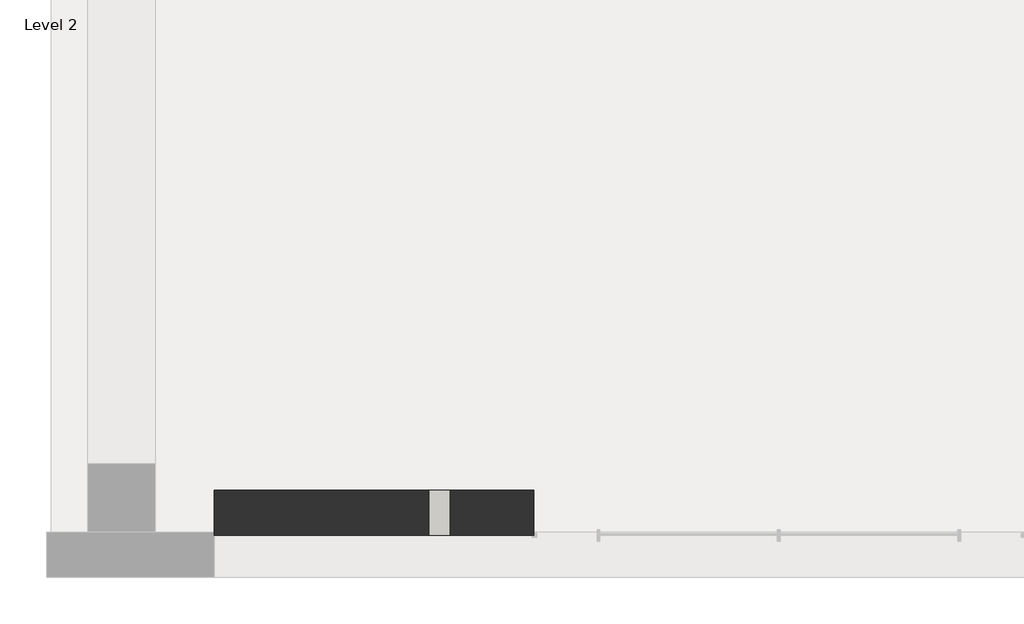
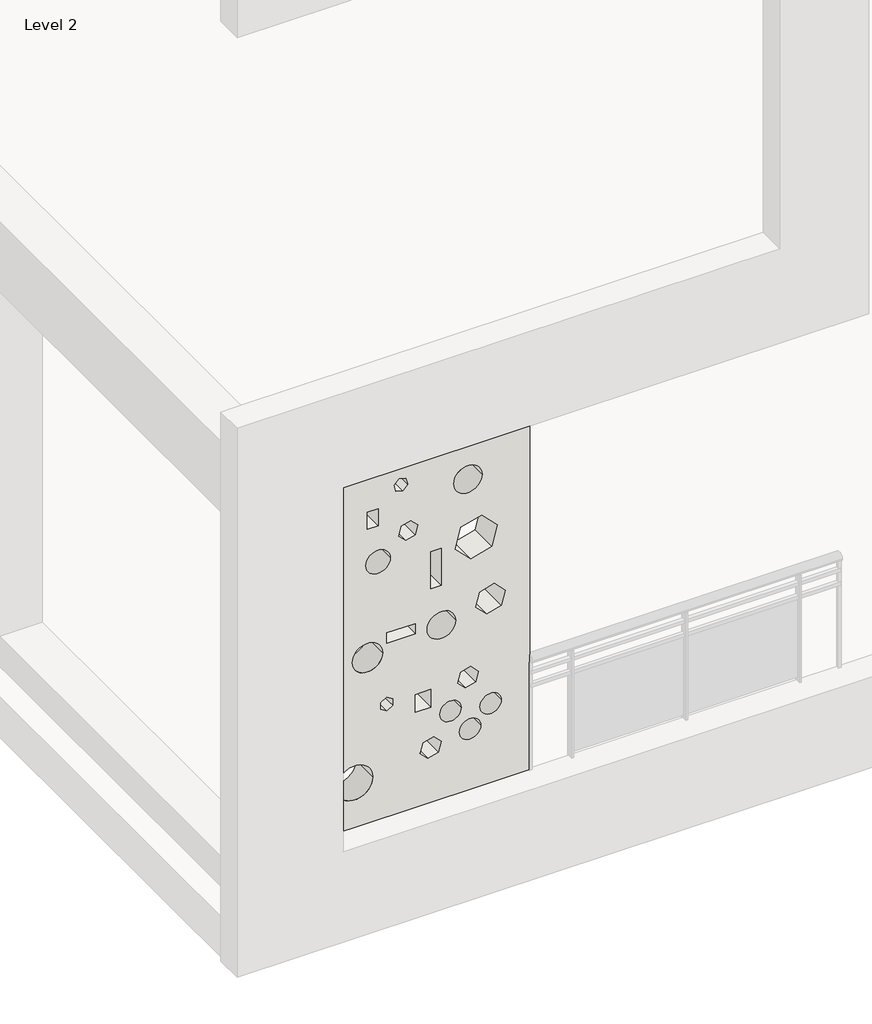
# One storey, part 1 of 2: 1 wall.
"""IFC4 building model written with IfcOpenShell, lengths in millimetres."""

from ifc_helpers import new_model, si_unit, frame, origin, place, context, project, spatial, polyline, circle_curve, element, save
from ifc_brep_helpers import plane_surface, revolved_surface, advanced_brep

model = new_model("IFC4")

# Units and contexts
model_context = context("Model", 3, world=origin())
ifc_project = project(units=[si_unit("LENGTHUNIT", "METRE", prefix="MILLI")], contexts=[model_context])

# Site, building, storey
site = spatial("IfcSite", under=ifc_project)
building = spatial("IfcBuilding", under=site)
storey = spatial("IfcBuildingStorey", under=building, Name="Level 2", Elevation=3657.6)

# Wall
placement = place(None, origin())
element("IfcWall", 1, ObjectType="Generic - 8\"", at=placement, inside=storey, context=model_context, shape_type="AdvancedBrep", body=[
    advanced_brep(
    [(-10102.8741466, 1544.2572776, 4341.7312703), (-8663.1307892, 1544.2572776, 4341.7312703), (-8663.1307892, 1544.2572776, 7084.9312703), (-10102.8741466, 1544.2572776, 7084.9312703), (-9743.8434722, 1544.2572776, 6685.8043423), (-9743.8434722, 1544.2572776, 6558.8043423), (-9820.0434722, 1544.2572776, 6558.8043423), (-9820.0434722, 1544.2572776, 6685.8043423), (-9292.3903484, 1544.2572776, 6229.9318449), (-9292.3903484, 1544.2572776, 5950.5318449), (-9368.5903484, 1544.2572776, 5950.5318449), (-9368.5903484, 1544.2572776, 6229.9318449), (-9479.1821198, 1544.2572776, 5728.8819866), (-9479.1821198, 1544.2572776, 5652.6819866), (-9682.3821198, 1544.2572776, 5652.6819866), (-9682.3821198, 1544.2572776, 5728.8819866), (-9368.5903484, 1544.2572776, 5193.0240889), (-9368.5903484, 1544.2572776, 5060.1832779), (-9479.1821198, 1544.2572776, 5060.1832779), (-9479.1821198, 1544.2572776, 5193.0240889), (-9001.4296873, 1544.2572776, 6685.8043423), (-9204.6296873, 1544.2572776, 6685.8043423), (-9656.9239941, 1544.2572776, 6287.1198438), (-9830.7629503, 1544.2572776, 6287.1198438), (-9190.7903484, 1544.2572776, 5652.6819866), (-9393.9903484, 1544.2572776, 5652.6819866), (-8970.421925, 1544.2572776, 5624.7908508), (-9046.621925, 1544.2572776, 5700.9908508), (-9018.7307892, 1544.2572776, 5805.0819866), (-8914.6396534, 1544.2572776, 5832.9731223), (-8838.4396534, 1544.2572776, 5756.7731223), (-8866.3307892, 1544.2572776, 5652.6819866), (-9084.3253885, 1544.2572776, 6079.9235581), (-9194.1390761, 1544.2572776, 6189.7372456), (-9153.9444768, 1544.2572776, 6339.7455325), (-9003.9361899, 1544.2572776, 6379.9401318), (-8894.1225023, 1544.2572776, 6270.1264443), (-8934.3171017, 1544.2572776, 6120.1181574), (-9630.1079092, 1544.2572776, 6823.2802275), (-9594.1868847, 1544.2572776, 6859.2012519), (-9545.1178527, 1544.2572776, 6846.0532445), (-9531.9698452, 1544.2572776, 6796.9842125), (-9567.8908697, 1544.2572776, 6761.063188), (-9616.9599017, 1544.2572776, 6774.2111955), (-9547.9311575, 1544.2572776, 6379.0943395), (-9598.2589461, 1544.2572776, 6429.4221281), (-9579.837697, 1544.2572776, 6498.1711658), (-9511.0886592, 1544.2572776, 6516.592415), (-9460.7608706, 1544.2572776, 6466.2646264), (-9479.1821198, 1544.2572776, 6397.5155887), (-9726.3762103, 1544.2572776, 5167.6240889), (-9726.3762103, 1544.2572776, 5218.4240889), (-9682.3821198, 1544.2572776, 5243.8240889), (-9638.3880293, 1544.2572776, 5218.4240889), (-9638.3880293, 1544.2572776, 5167.6240889), (-9682.3821198, 1544.2572776, 5142.2240889), (-9121.9120367, 1544.2572776, 5119.4205409), (-9175.7935734, 1544.2572776, 5173.3020776), (-9156.0715622, 1544.2572776, 5246.9056256), (-9082.4680142, 1544.2572776, 5266.6276368), (-9028.5864775, 1544.2572776, 5212.7461001), (-9048.3084887, 1544.2572776, 5139.1425521), (-9388.391626, 1544.2572776, 4681.4839037), (-9442.4897226, 1544.2572776, 4735.5820003), (-9422.688445, 1544.2572776, 4809.4813745), (-9348.7890707, 1544.2572776, 4829.2826522), (-9294.6909741, 1544.2572776, 4775.1845556), (-9314.4922518, 1544.2572776, 4701.2851813), (-9011.4676213, 1544.2572776, 4798.8655131), (-9163.8676213, 1544.2572776, 4798.8655131), (-8864.8322569, 1544.2572776, 4938.5407612), (-9017.2322569, 1544.2572776, 4938.5407612), (-9151.0988797, 1544.2572776, 4981.0816577), (-9303.4988797, 1544.2572776, 4981.0816577), (-9782.375451, 1544.2572776, 4678.6434787), (-10039.5887886, 1544.2572776, 4678.6434787), (-9712.2803987, 1544.2572776, 5590.3709003), (-9927.8065456, 1544.2572776, 5590.3709003), (-10102.8741466, 1747.4572776, 4341.7312703), (-10102.8741466, 1747.4572776, 7084.9312703), (-8663.1307892, 1747.4572776, 7084.9312703), (-8663.1307892, 1747.4572776, 4341.7312703), (-9743.8434722, 1747.4572776, 6685.8043423), (-9820.0434722, 1747.4572776, 6685.8043423), (-9820.0434722, 1747.4572776, 6558.8043423), (-9743.8434722, 1747.4572776, 6558.8043423), (-9292.3903484, 1747.4572776, 6229.9318449), (-9368.5903484, 1747.4572776, 6229.9318449), (-9368.5903484, 1747.4572776, 5950.5318449), (-9292.3903484, 1747.4572776, 5950.5318449), (-9479.1821198, 1747.4572776, 5728.8819866), (-9682.3821198, 1747.4572776, 5728.8819866), (-9682.3821198, 1747.4572776, 5652.6819866), (-9479.1821198, 1747.4572776, 5652.6819866), (-9368.5903484, 1747.4572776, 5193.0240889), (-9479.1821198, 1747.4572776, 5193.0240889), (-9479.1821198, 1747.4572776, 5060.1832779), (-9368.5903484, 1747.4572776, 5060.1832779), (-9001.4296873, 1747.4572776, 6685.8043423), (-9204.6296873, 1747.4572776, 6685.8043423), (-9656.9239941, 1747.4572776, 6287.1198438), (-9830.7629503, 1747.4572776, 6287.1198438), (-9190.7903484, 1747.4572776, 5652.6819866), (-9393.9903484, 1747.4572776, 5652.6819866), (-8970.421925, 1747.4572776, 5624.7908508), (-8866.3307892, 1747.4572776, 5652.6819866), (-8838.4396534, 1747.4572776, 5756.7731223), (-8914.6396534, 1747.4572776, 5832.9731223), (-9018.7307892, 1747.4572776, 5805.0819866), (-9046.621925, 1747.4572776, 5700.9908508), (-9084.3253885, 1747.4572776, 6079.9235581), (-8934.3171017, 1747.4572776, 6120.1181574), (-8894.1225023, 1747.4572776, 6270.1264443), (-9003.9361899, 1747.4572776, 6379.9401318), (-9153.9444768, 1747.4572776, 6339.7455325), (-9194.1390761, 1747.4572776, 6189.7372456), (-9630.1079092, 1747.4572776, 6823.2802275), (-9616.9599017, 1747.4572776, 6774.2111955), (-9567.8908697, 1747.4572776, 6761.063188), (-9531.9698452, 1747.4572776, 6796.9842125), (-9545.1178527, 1747.4572776, 6846.0532445), (-9594.1868847, 1747.4572776, 6859.2012519), (-9547.9311575, 1747.4572776, 6379.0943395), (-9479.1821198, 1747.4572776, 6397.5155887), (-9460.7608706, 1747.4572776, 6466.2646264), (-9511.0886592, 1747.4572776, 6516.592415), (-9579.837697, 1747.4572776, 6498.1711658), (-9598.2589461, 1747.4572776, 6429.4221281), (-9726.3762103, 1747.4572776, 5167.6240889), (-9682.3821198, 1747.4572776, 5142.2240889), (-9638.3880293, 1747.4572776, 5167.6240889), (-9638.3880293, 1747.4572776, 5218.4240889), (-9682.3821198, 1747.4572776, 5243.8240889), (-9726.3762103, 1747.4572776, 5218.4240889), (-9121.9120367, 1747.4572776, 5119.4205409), (-9048.3084887, 1747.4572776, 5139.1425521), (-9028.5864775, 1747.4572776, 5212.7461001), (-9082.4680142, 1747.4572776, 5266.6276368), (-9156.0715622, 1747.4572776, 5246.9056256), (-9175.7935734, 1747.4572776, 5173.3020776), (-9388.391626, 1747.4572776, 4681.4839037), (-9314.4922518, 1747.4572776, 4701.2851813), (-9294.6909741, 1747.4572776, 4775.1845556), (-9348.7890707, 1747.4572776, 4829.2826522), (-9422.688445, 1747.4572776, 4809.4813745), (-9442.4897226, 1747.4572776, 4735.5820003), (-9011.4676213, 1747.4572776, 4798.8655131), (-9163.8676213, 1747.4572776, 4798.8655131), (-8864.8322569, 1747.4572776, 4938.5407612), (-9017.2322569, 1747.4572776, 4938.5407612), (-9151.0988797, 1747.4572776, 4981.0816577), (-9303.4988797, 1747.4572776, 4981.0816577), (-9782.375451, 1747.4572776, 4678.6434787), (-10039.5887886, 1747.4572776, 4678.6434787), (-9712.2803987, 1747.4572776, 5590.3709003), (-9927.8065456, 1747.4572776, 5590.3709003), (-10102.8741466, 1558.4652184, 4341.7312703), (-10102.8741466, 1558.4652184, 7084.9312703)],
    [
        (0, 1),
        (1, 2),
        (2, 3),
        (3, 0),
        (4, 5),
        (5, 6),
        (6, 7),
        (7, 4),
        (8, 9),
        (9, 10),
        (10, 11),
        (11, 8),
        (12, 13),
        (13, 14),
        (14, 15),
        (15, 12),
        (16, 17),
        (17, 18),
        (18, 19),
        (19, 16),
        (20, 21, circle_curve(frame((-9103.0296873, 1544.2572776, 6685.8043423), z_axis=(0.0, 1.0, 0.0), x_axis=(-1.0, 0.0, 0.0)), 101.6)),
        (21, 20, circle_curve(frame((-9103.0296873, 1544.2572776, 6685.8043423), z_axis=(0.0, 1.0, 0.0), x_axis=(-1.0, 0.0, 0.0)), 101.6)),
        (22, 23, circle_curve(frame((-9743.8434722, 1544.2572776, 6287.1198438), z_axis=(0.0, 1.0, 0.0), x_axis=(-1.0, 0.0, 0.0)), 86.9194781)),
        (23, 22, circle_curve(frame((-9743.8434722, 1544.2572776, 6287.1198438), z_axis=(0.0, 1.0, 0.0), x_axis=(-1.0, 0.0, 0.0)), 86.9194781)),
        (24, 25, circle_curve(frame((-9292.3903484, 1544.2572776, 5652.6819866), z_axis=(0.0, 1.0, 0.0), x_axis=(-1.0, 0.0, 0.0)), 101.6)),
        (25, 24, circle_curve(frame((-9292.3903484, 1544.2572776, 5652.6819866), z_axis=(0.0, 1.0, 0.0), x_axis=(-1.0, 0.0, 0.0)), 101.6)),
        (26, 27),
        (27, 28),
        (28, 29),
        (29, 30),
        (30, 31),
        (31, 26),
        (32, 33),
        (33, 34),
        (34, 35),
        (35, 36),
        (36, 37),
        (37, 32),
        (38, 39),
        (39, 40),
        (40, 41),
        (41, 42),
        (42, 43),
        (43, 38),
        (44, 45),
        (45, 46),
        (46, 47),
        (47, 48),
        (48, 49),
        (49, 44),
        (50, 51),
        (51, 52),
        (52, 53),
        (53, 54),
        (54, 55),
        (55, 50),
        (56, 57),
        (57, 58),
        (58, 59),
        (59, 60),
        (60, 61),
        (61, 56),
        (62, 63),
        (63, 64),
        (64, 65),
        (65, 66),
        (66, 67),
        (67, 62),
        (68, 69, circle_curve(frame((-9087.6676213, 1544.2572776, 4798.8655131), z_axis=(0.0, 1.0, 0.0), x_axis=(-1.0, 0.0, 0.0)), 76.2)),
        (69, 68, circle_curve(frame((-9087.6676213, 1544.2572776, 4798.8655131), z_axis=(0.0, 1.0, 0.0), x_axis=(-1.0, 0.0, 0.0)), 76.2)),
        (70, 71, circle_curve(frame((-8941.0322569, 1544.2572776, 4938.5407612), z_axis=(0.0, 1.0, 0.0), x_axis=(-1.0, 0.0, 0.0)), 76.2)),
        (71, 70, circle_curve(frame((-8941.0322569, 1544.2572776, 4938.5407612), z_axis=(0.0, 1.0, 0.0), x_axis=(-1.0, 0.0, 0.0)), 76.2)),
        (72, 73, circle_curve(frame((-9227.2988797, 1544.2572776, 4981.0816577), z_axis=(0.0, 1.0, 0.0), x_axis=(-1.0, 0.0, 0.0)), 76.2)),
        (73, 72, circle_curve(frame((-9227.2988797, 1544.2572776, 4981.0816577), z_axis=(0.0, 1.0, 0.0), x_axis=(-1.0, 0.0, 0.0)), 76.2)),
        (74, 75, circle_curve(frame((-9910.9821198, 1544.2572776, 4678.6434787), z_axis=(0.0, 1.0, 0.0), x_axis=(-1.0, 0.0, 0.0)), 128.6066688)),
        (75, 74, circle_curve(frame((-9910.9821198, 1544.2572776, 4678.6434787), z_axis=(0.0, 1.0, 0.0), x_axis=(-1.0, 0.0, 0.0)), 128.6066688)),
        (76, 77, circle_curve(frame((-9820.0434722, 1544.2572776, 5590.3709003), z_axis=(0.0, 1.0, 0.0), x_axis=(-1.0, 0.0, 0.0)), 107.7630735)),
        (77, 76, circle_curve(frame((-9820.0434722, 1544.2572776, 5590.3709003), z_axis=(0.0, 1.0, 0.0), x_axis=(-1.0, 0.0, 0.0)), 107.7630735)),
        (78, 79),
        (79, 80),
        (80, 81),
        (81, 78),
        (82, 83),
        (83, 84),
        (84, 85),
        (85, 82),
        (86, 87),
        (87, 88),
        (88, 89),
        (89, 86),
        (90, 91),
        (91, 92),
        (92, 93),
        (93, 90),
        (94, 95),
        (95, 96),
        (96, 97),
        (97, 94),
        (98, 99, circle_curve(frame((-9103.0296873, 1747.4572776, 6685.8043423), z_axis=(0.0, -1.0, 0.0), x_axis=(-1.0, 0.0, 0.0)), 101.6)),
        (99, 98, circle_curve(frame((-9103.0296873, 1747.4572776, 6685.8043423), z_axis=(0.0, -1.0, 0.0), x_axis=(-1.0, 0.0, 0.0)), 101.6)),
        (100, 101, circle_curve(frame((-9743.8434722, 1747.4572776, 6287.1198438), z_axis=(0.0, -1.0, 0.0), x_axis=(-1.0, 0.0, 0.0)), 86.9194781)),
        (101, 100, circle_curve(frame((-9743.8434722, 1747.4572776, 6287.1198438), z_axis=(0.0, -1.0, 0.0), x_axis=(-1.0, 0.0, 0.0)), 86.9194781)),
        (102, 103, circle_curve(frame((-9292.3903484, 1747.4572776, 5652.6819866), z_axis=(0.0, -1.0, 0.0), x_axis=(-1.0, 0.0, 0.0)), 101.6)),
        (103, 102, circle_curve(frame((-9292.3903484, 1747.4572776, 5652.6819866), z_axis=(0.0, -1.0, 0.0), x_axis=(-1.0, 0.0, 0.0)), 101.6)),
        (104, 105),
        (105, 106),
        (106, 107),
        (107, 108),
        (108, 109),
        (109, 104),
        (110, 111),
        (111, 112),
        (112, 113),
        (113, 114),
        (114, 115),
        (115, 110),
        (116, 117),
        (117, 118),
        (118, 119),
        (119, 120),
        (120, 121),
        (121, 116),
        (122, 123),
        (123, 124),
        (124, 125),
        (125, 126),
        (126, 127),
        (127, 122),
        (128, 129),
        (129, 130),
        (130, 131),
        (131, 132),
        (132, 133),
        (133, 128),
        (134, 135),
        (135, 136),
        (136, 137),
        (137, 138),
        (138, 139),
        (139, 134),
        (140, 141),
        (141, 142),
        (142, 143),
        (143, 144),
        (144, 145),
        (145, 140),
        (146, 147, circle_curve(frame((-9087.6676213, 1747.4572776, 4798.8655131), z_axis=(0.0, -1.0, 0.0), x_axis=(-1.0, 0.0, 0.0)), 76.2)),
        (147, 146, circle_curve(frame((-9087.6676213, 1747.4572776, 4798.8655131), z_axis=(0.0, -1.0, 0.0), x_axis=(-1.0, 0.0, 0.0)), 76.2)),
        (148, 149, circle_curve(frame((-8941.0322569, 1747.4572776, 4938.5407612), z_axis=(0.0, -1.0, 0.0), x_axis=(-1.0, 0.0, 0.0)), 76.2)),
        (149, 148, circle_curve(frame((-8941.0322569, 1747.4572776, 4938.5407612), z_axis=(0.0, -1.0, 0.0), x_axis=(-1.0, 0.0, 0.0)), 76.2)),
        (150, 151, circle_curve(frame((-9227.2988797, 1747.4572776, 4981.0816577), z_axis=(0.0, -1.0, 0.0), x_axis=(-1.0, 0.0, 0.0)), 76.2)),
        (151, 150, circle_curve(frame((-9227.2988797, 1747.4572776, 4981.0816577), z_axis=(0.0, -1.0, 0.0), x_axis=(-1.0, 0.0, 0.0)), 76.2)),
        (152, 153, circle_curve(frame((-9910.9821198, 1747.4572776, 4678.6434787), z_axis=(0.0, -1.0, 0.0), x_axis=(-1.0, 0.0, 0.0)), 128.6066688)),
        (153, 152, circle_curve(frame((-9910.9821198, 1747.4572776, 4678.6434787), z_axis=(0.0, -1.0, 0.0), x_axis=(-1.0, 0.0, 0.0)), 128.6066688)),
        (154, 155, circle_curve(frame((-9820.0434722, 1747.4572776, 5590.3709003), z_axis=(0.0, -1.0, 0.0), x_axis=(-1.0, 0.0, 0.0)), 107.7630735)),
        (155, 154, circle_curve(frame((-9820.0434722, 1747.4572776, 5590.3709003), z_axis=(0.0, -1.0, 0.0), x_axis=(-1.0, 0.0, 0.0)), 107.7630735)),
        (0, 156),
        (156, 78),
        (81, 1),
        (80, 2),
        (79, 157),
        (157, 3),
        (4, 82),
        (85, 5),
        (84, 6),
        (83, 7),
        (8, 86),
        (89, 9),
        (88, 10),
        (87, 11),
        (12, 90),
        (93, 13),
        (92, 14),
        (91, 15),
        (16, 94),
        (97, 17),
        (96, 18),
        (95, 19),
        (20, 98),
        (99, 21),
        (22, 100),
        (101, 23),
        (24, 102),
        (103, 25),
        (26, 104),
        (109, 27),
        (108, 28),
        (107, 29),
        (106, 30),
        (105, 31),
        (32, 110),
        (115, 33),
        (114, 34),
        (113, 35),
        (112, 36),
        (111, 37),
        (38, 116),
        (121, 39),
        (120, 40),
        (119, 41),
        (118, 42),
        (117, 43),
        (44, 122),
        (127, 45),
        (126, 46),
        (125, 47),
        (124, 48),
        (123, 49),
        (50, 128),
        (133, 51),
        (132, 52),
        (131, 53),
        (130, 54),
        (129, 55),
        (56, 134),
        (139, 57),
        (138, 58),
        (137, 59),
        (136, 60),
        (135, 61),
        (62, 140),
        (145, 63),
        (144, 64),
        (143, 65),
        (142, 66),
        (141, 67),
        (68, 146),
        (147, 69),
        (70, 148),
        (149, 71),
        (72, 150),
        (151, 73),
        (74, 152),
        (153, 75),
        (76, 154),
        (155, 77),
    ],
    [
        plane_surface(frame((-10102.8741466, 1544.2572776, 4341.7312703), z_axis=(0.0, -1.0, 0.0), x_axis=(1.0, 0.0, 0.0))),
        plane_surface(frame((-10102.8741466, 1747.4572776, 4341.7312703), z_axis=(0.0, 1.0, 0.0), x_axis=(-1.0, 0.0, 0.0))),
        plane_surface(frame((-10102.8741466, 1544.2572776, 4341.7312703), z_axis=(0.0, 0.0, -1.0), x_axis=(0.0, 1.0, 0.0))),
        plane_surface(frame((-8663.1307892, 1544.2572776, 4341.7312703), z_axis=(1.0, 0.0, 0.0), x_axis=(0.0, 1.0, 0.0))),
        plane_surface(frame((-8663.1307892, 1544.2572776, 7084.9312703), z_axis=(0.0, 0.0, 1.0), x_axis=(0.0, 1.0, 0.0))),
        plane_surface(frame((-10102.8741466, 1544.2572776, 7084.9312703), z_axis=(-1.0, 0.0, 0.0), x_axis=(0.0, 1.0, 0.0))),
        plane_surface(frame((-9743.8434722, 1544.2572776, 6685.8043423), z_axis=(-1.0, 0.0, 0.0), x_axis=(0.0, 1.0, 0.0))),
        plane_surface(frame((-9743.8434722, 1544.2572776, 6558.8043423), z_axis=(0.0, 0.0, 1.0), x_axis=(0.0, 1.0, 0.0))),
        plane_surface(frame((-9820.0434722, 1544.2572776, 6558.8043423), z_axis=(1.0, 0.0, 0.0), x_axis=(0.0, 1.0, 0.0))),
        plane_surface(frame((-9820.0434722, 1544.2572776, 6685.8043423), z_axis=(0.0, 0.0, -1.0), x_axis=(0.0, 1.0, 0.0))),
        plane_surface(frame((-9292.3903484, 1544.2572776, 6229.9318449), z_axis=(-1.0, 0.0, 0.0), x_axis=(0.0, 1.0, 0.0))),
        plane_surface(frame((-9292.3903484, 1544.2572776, 5950.5318449), z_axis=(0.0, 0.0, 1.0), x_axis=(0.0, 1.0, 0.0))),
        plane_surface(frame((-9368.5903484, 1544.2572776, 5950.5318449), z_axis=(1.0, 0.0, 0.0), x_axis=(0.0, 1.0, 0.0))),
        plane_surface(frame((-9368.5903484, 1544.2572776, 6229.9318449), z_axis=(0.0, 0.0, -1.0), x_axis=(0.0, 1.0, 0.0))),
        plane_surface(frame((-9479.1821198, 1544.2572776, 5728.8819866), z_axis=(-1.0, 0.0, 0.0), x_axis=(0.0, 1.0, 0.0))),
        plane_surface(frame((-9479.1821198, 1544.2572776, 5652.6819866), z_axis=(0.0, 0.0, 1.0), x_axis=(0.0, 1.0, 0.0))),
        plane_surface(frame((-9682.3821198, 1544.2572776, 5652.6819866), z_axis=(1.0, 0.0, 0.0), x_axis=(0.0, 1.0, 0.0))),
        plane_surface(frame((-9682.3821198, 1544.2572776, 5728.8819866), z_axis=(0.0, 0.0, -1.0), x_axis=(0.0, 1.0, 0.0))),
        plane_surface(frame((-9368.5903484, 1544.2572776, 5193.0240889), z_axis=(-1.0, 0.0, 0.0), x_axis=(0.0, 1.0, 0.0))),
        plane_surface(frame((-9368.5903484, 1544.2572776, 5060.1832779), z_axis=(0.0, 0.0, 1.0), x_axis=(0.0, 1.0, 0.0))),
        plane_surface(frame((-9479.1821198, 1544.2572776, 5060.1832779), z_axis=(1.0, 0.0, 0.0), x_axis=(0.0, 1.0, 0.0))),
        plane_surface(frame((-9479.1821198, 1544.2572776, 5193.0240889), z_axis=(0.0, 0.0, -1.0), x_axis=(0.0, 1.0, 0.0))),
        revolved_surface(polyline([(-9204.629687300001, 1747.4572776, 6685.8043423), (-9204.629687300001, 1544.2572776, 6685.8043423)]), (-9103.0296873, 1645.8572776, 6685.8043423), (0.0, 1.0, 0.0)),
        revolved_surface(polyline([(-9830.7629503, 1747.4572776, 6287.1198438), (-9830.7629503, 1544.2572776, 6287.1198438)]), (-9743.8434722, 1645.8572776, 6287.1198438), (0.0, 1.0, 0.0)),
        revolved_surface(polyline([(-9393.9903484, 1747.4572776, 5652.6819866), (-9393.9903484, 1544.2572776, 5652.6819866)]), (-9292.3903484, 1645.8572776, 5652.6819866), (0.0, 1.0, 0.0)),
        plane_surface(frame((-8970.421925, 1544.2572776, 5624.7908508), z_axis=(0.7071067811865426, 0.0, 0.7071067811865526), x_axis=(0.0, 1.0, 0.0))),
        plane_surface(frame((-9046.621925, 1544.2572776, 5700.9908508), z_axis=(0.9659258262890714, 0.0, -0.25881904510250914), x_axis=(0.0, 1.0, 0.0))),
        plane_surface(frame((-9018.7307892, 1544.2572776, 5805.0819866), z_axis=(0.25881904510252784, 0.0, -0.9659258262890664), x_axis=(0.0, 1.0, 0.0))),
        plane_surface(frame((-8914.6396534, 1544.2572776, 5832.9731223), z_axis=(-0.7071067811865375, 0.0, -0.7071067811865576), x_axis=(0.0, 1.0, 0.0))),
        plane_surface(frame((-8838.4396534, 1544.2572776, 5756.7731223), z_axis=(-0.9659258262890714, 0.0, 0.25881904510250914), x_axis=(0.0, 1.0, 0.0))),
        plane_surface(frame((-8866.3307892, 1544.2572776, 5652.6819866), z_axis=(-0.25881904510252535, 0.0, 0.9659258262890671), x_axis=(0.0, 1.0, 0.0))),
        plane_surface(frame((-9084.3253885, 1544.2572776, 6079.9235581), z_axis=(0.707106781186544, 0.0, 0.707106781186551), x_axis=(0.0, 1.0, 0.0))),
        plane_surface(frame((-9194.1390761, 1544.2572776, 6189.7372456), z_axis=(0.9659258262890703, 0.0, -0.2588190451025133), x_axis=(0.0, 1.0, 0.0))),
        plane_surface(frame((-9153.9444768, 1544.2572776, 6339.7455325), z_axis=(0.2588190451025328, 0.0, -0.9659258262890651), x_axis=(0.0, 1.0, 0.0))),
        plane_surface(frame((-9003.9361899, 1544.2572776, 6379.9401318), z_axis=(-0.7071067811865406, 0.0, -0.7071067811865545), x_axis=(0.0, 1.0, 0.0))),
        plane_surface(frame((-8894.1225023, 1544.2572776, 6270.1264443), z_axis=(-0.9659258262890713, 0.0, 0.2588190451025098), x_axis=(0.0, 1.0, 0.0))),
        plane_surface(frame((-8934.3171017, 1544.2572776, 6120.1181574), z_axis=(-0.2588190451025263, 0.0, 0.9659258262890669), x_axis=(0.0, 1.0, 0.0))),
        plane_surface(frame((-9630.1079092, 1544.2572776, 6823.2802275), z_axis=(0.7071067811865582, 0.0, -0.7071067811865369), x_axis=(0.0, 1.0, 0.0))),
        plane_surface(frame((-9594.1868847, 1544.2572776, 6859.2012519), z_axis=(-0.2588190451025169, 0.0, -0.9659258262890693), x_axis=(0.0, 1.0, 0.0))),
        plane_surface(frame((-9545.1178527, 1544.2572776, 6846.0532445), z_axis=(-0.965925826289064, 0.0, -0.25881904510253684), x_axis=(0.0, 1.0, 0.0))),
        plane_surface(frame((-9531.9698452, 1544.2572776, 6796.9842125), z_axis=(-0.7071067811865582, 0.0, 0.7071067811865369), x_axis=(0.0, 1.0, 0.0))),
        plane_surface(frame((-9567.8908697, 1544.2572776, 6761.063188), z_axis=(0.2588190451025169, 0.0, 0.9659258262890693), x_axis=(0.0, 1.0, 0.0))),
        plane_surface(frame((-9616.9599017, 1544.2572776, 6774.2111955), z_axis=(0.965925826289064, 0.0, 0.25881904510253684), x_axis=(0.0, 1.0, 0.0))),
        plane_surface(frame((-9547.9311575, 1544.2572776, 6379.0943395), z_axis=(0.7071067811865399, 0.0, 0.7071067811865551), x_axis=(0.0, 1.0, 0.0))),
        plane_surface(frame((-9598.2589461, 1544.2572776, 6429.4221281), z_axis=(0.9659258262890762, 0.0, -0.2588190451024913), x_axis=(0.0, 1.0, 0.0))),
        plane_surface(frame((-9579.837697, 1544.2572776, 6498.1711658), z_axis=(0.25881904510253395, 0.0, -0.9659258262890648), x_axis=(0.0, 1.0, 0.0))),
        plane_surface(frame((-9511.0886592, 1544.2572776, 6516.592415), z_axis=(-0.7071067811865399, 0.0, -0.7071067811865551), x_axis=(0.0, 1.0, 0.0))),
        plane_surface(frame((-9460.7608706, 1544.2572776, 6466.2646264), z_axis=(-0.9659258262890762, 0.0, 0.2588190451024913), x_axis=(0.0, 1.0, 0.0))),
        plane_surface(frame((-9479.1821198, 1544.2572776, 6397.5155887), z_axis=(-0.25881904510253395, 0.0, 0.9659258262890648), x_axis=(0.0, 1.0, 0.0))),
        plane_surface(frame((-9726.3762103, 1544.2572776, 5167.6240889), z_axis=(1.0, 0.0, 0.0), x_axis=(0.0, 1.0, 0.0))),
        plane_surface(frame((-9726.3762103, 1544.2572776, 5218.4240889), z_axis=(0.4999999999999623, 0.0, -0.8660254037844605), x_axis=(0.0, 1.0, 0.0))),
        plane_surface(frame((-9682.3821198, 1544.2572776, 5243.8240889), z_axis=(-0.5000000000000288, 0.0, -0.8660254037844222), x_axis=(0.0, 1.0, 0.0))),
        plane_surface(frame((-9638.3880293, 1544.2572776, 5218.4240889), z_axis=(-1.0, 0.0, 0.0), x_axis=(0.0, 1.0, 0.0))),
        plane_surface(frame((-9638.3880293, 1544.2572776, 5167.6240889), z_axis=(-0.4999999999999783, 0.0, 0.8660254037844513), x_axis=(0.0, 1.0, 0.0))),
        plane_surface(frame((-9682.3821198, 1544.2572776, 5142.2240889), z_axis=(0.5000000000000288, 0.0, 0.8660254037844222), x_axis=(0.0, 1.0, 0.0))),
        plane_surface(frame((-9121.9120367, 1544.2572776, 5119.4205409), z_axis=(0.7071067811865405, 0.0, 0.7071067811865547), x_axis=(0.0, 1.0, 0.0))),
        plane_surface(frame((-9175.7935734, 1544.2572776, 5173.3020776), z_axis=(0.9659258262890702, 0.0, -0.25881904510251386), x_axis=(0.0, 1.0, 0.0))),
        plane_surface(frame((-9156.0715622, 1544.2572776, 5246.9056256), z_axis=(0.2588190451025271, 0.0, -0.9659258262890666), x_axis=(0.0, 1.0, 0.0))),
        plane_surface(frame((-9082.4680142, 1544.2572776, 5266.6276368), z_axis=(-0.7071067811865405, 0.0, -0.7071067811865547), x_axis=(0.0, 1.0, 0.0))),
        plane_surface(frame((-9028.5864775, 1544.2572776, 5212.7461001), z_axis=(-0.9659258262890702, 0.0, 0.25881904510251386), x_axis=(0.0, 1.0, 0.0))),
        plane_surface(frame((-9048.3084887, 1544.2572776, 5139.1425521), z_axis=(-0.2588190451025271, 0.0, 0.9659258262890666), x_axis=(0.0, 1.0, 0.0))),
        plane_surface(frame((-9388.391626, 1544.2572776, 4681.4839037), z_axis=(0.7071067811865405, 0.0, 0.7071067811865547), x_axis=(0.0, 1.0, 0.0))),
        plane_surface(frame((-9442.4897226, 1544.2572776, 4735.5820003), z_axis=(0.9659258262890724, 0.0, -0.25881904510250564), x_axis=(0.0, 1.0, 0.0))),
        plane_surface(frame((-9422.688445, 1544.2572776, 4809.4813745), z_axis=(0.25881904510253556, 0.0, -0.9659258262890643), x_axis=(0.0, 1.0, 0.0))),
        plane_surface(frame((-9348.7890707, 1544.2572776, 4829.2826522), z_axis=(-0.7071067811865405, 0.0, -0.7071067811865547), x_axis=(0.0, 1.0, 0.0))),
        plane_surface(frame((-9294.6909741, 1544.2572776, 4775.1845556), z_axis=(-0.9659258262890754, 0.0, 0.2588190451024942), x_axis=(0.0, 1.0, 0.0))),
        plane_surface(frame((-9314.4922518, 1544.2572776, 4701.2851813), z_axis=(-0.2588190451025386, 0.0, 0.9659258262890635), x_axis=(0.0, 1.0, 0.0))),
        revolved_surface(polyline([(-9163.8676213, 1747.4572776, 4798.8655131), (-9163.8676213, 1544.2572776, 4798.8655131)]), (-9087.6676213, 1645.8572776, 4798.8655131), (0.0, 1.0, 0.0)),
        revolved_surface(polyline([(-9017.2322569, 1747.4572776, 4938.5407612), (-9017.2322569, 1544.2572776, 4938.5407612)]), (-8941.0322569, 1645.8572776, 4938.5407612), (0.0, 1.0, 0.0)),
        revolved_surface(polyline([(-9303.4988797, 1747.4572776, 4981.0816577), (-9303.4988797, 1544.2572776, 4981.0816577)]), (-9227.2988797, 1645.8572776, 4981.0816577), (0.0, 1.0, 0.0)),
        revolved_surface(polyline([(-10039.5887886, 1747.4572776, 4678.6434787), (-10039.5887886, 1544.2572776, 4678.6434787)]), (-9910.9821198, 1645.8572776, 4678.6434787), (0.0, 1.0, 0.0)),
        revolved_surface(polyline([(-9927.806545700001, 1747.4572776, 5590.3709003), (-9927.806545700001, 1544.2572776, 5590.3709003)]), (-9820.0434722, 1645.8572776, 5590.3709003), (0.0, 1.0, 0.0)),
    ],
    [
        (0, [[1, 2, 3, 4], [5, 6, 7, 8], [9, 10, 11, 12], [13, 14, 15, 16], [17, 18, 19, 20], [21, 22], [23, 24], [25, 26], [27, 28, 29, 30, 31, 32], [33, 34, 35, 36, 37, 38], [39, 40, 41, 42, 43, 44], [45, 46, 47, 48, 49, 50], [51, 52, 53, 54, 55, 56], [57, 58, 59, 60, 61, 62], [63, 64, 65, 66, 67, 68], [69, 70], [71, 72], [73, 74], [75, 76], [77, 78]]),
        (1, [[79, 80, 81, 82], [83, 84, 85, 86], [87, 88, 89, 90], [91, 92, 93, 94], [95, 96, 97, 98], [99, 100], [101, 102], [103, 104], [105, 106, 107, 108, 109, 110], [111, 112, 113, 114, 115, 116], [117, 118, 119, 120, 121, 122], [123, 124, 125, 126, 127, 128], [129, 130, 131, 132, 133, 134], [135, 136, 137, 138, 139, 140], [141, 142, 143, 144, 145, 146], [147, 148], [149, 150], [151, 152], [153, 154], [155, 156]]),
        (2, [[-1, 157, 158, -82, 159]]),
        (3, [[-2, -159, -81, 160]]),
        (4, [[-3, -160, -80, 161, 162]]),
        (5, [[-4, -162, -161, -79, -158, -157]]),
        (6, [[-5, 163, -86, 164]]),
        (7, [[-6, -164, -85, 165]]),
        (8, [[-7, -165, -84, 166]]),
        (9, [[-8, -166, -83, -163]]),
        (10, [[-9, 167, -90, 168]]),
        (11, [[-10, -168, -89, 169]]),
        (12, [[-11, -169, -88, 170]]),
        (13, [[-12, -170, -87, -167]]),
        (14, [[-13, 171, -94, 172]]),
        (15, [[-14, -172, -93, 173]]),
        (16, [[-15, -173, -92, 174]]),
        (17, [[-16, -174, -91, -171]]),
        (18, [[-17, 175, -98, 176]]),
        (19, [[-18, -176, -97, 177]]),
        (20, [[-19, -177, -96, 178]]),
        (21, [[-20, -178, -95, -175]]),
        (22, [[-21, 179, -100, 180]]),
        (22, [[-22, -180, -99, -179]]),
        (23, [[-23, 181, -102, 182]]),
        (23, [[-24, -182, -101, -181]]),
        (24, [[-25, 183, -104, 184]]),
        (24, [[-26, -184, -103, -183]]),
        (25, [[-27, 185, -110, 186]]),
        (26, [[-28, -186, -109, 187]]),
        (27, [[-29, -187, -108, 188]]),
        (28, [[-30, -188, -107, 189]]),
        (29, [[-31, -189, -106, 190]]),
        (30, [[-32, -190, -105, -185]]),
        (31, [[-33, 191, -116, 192]]),
        (32, [[-34, -192, -115, 193]]),
        (33, [[-35, -193, -114, 194]]),
        (34, [[-36, -194, -113, 195]]),
        (35, [[-37, -195, -112, 196]]),
        (36, [[-38, -196, -111, -191]]),
        (37, [[-39, 197, -122, 198]]),
        (38, [[-40, -198, -121, 199]]),
        (39, [[-41, -199, -120, 200]]),
        (40, [[-42, -200, -119, 201]]),
        (41, [[-43, -201, -118, 202]]),
        (42, [[-44, -202, -117, -197]]),
        (43, [[-45, 203, -128, 204]]),
        (44, [[-46, -204, -127, 205]]),
        (45, [[-47, -205, -126, 206]]),
        (46, [[-48, -206, -125, 207]]),
        (47, [[-49, -207, -124, 208]]),
        (48, [[-50, -208, -123, -203]]),
        (49, [[-51, 209, -134, 210]]),
        (50, [[-52, -210, -133, 211]]),
        (51, [[-53, -211, -132, 212]]),
        (52, [[-54, -212, -131, 213]]),
        (53, [[-55, -213, -130, 214]]),
        (54, [[-56, -214, -129, -209]]),
        (55, [[-57, 215, -140, 216]]),
        (56, [[-58, -216, -139, 217]]),
        (57, [[-59, -217, -138, 218]]),
        (58, [[-60, -218, -137, 219]]),
        (59, [[-61, -219, -136, 220]]),
        (60, [[-62, -220, -135, -215]]),
        (61, [[-63, 221, -146, 222]]),
        (62, [[-64, -222, -145, 223]]),
        (63, [[-65, -223, -144, 224]]),
        (64, [[-66, -224, -143, 225]]),
        (65, [[-67, -225, -142, 226]]),
        (66, [[-68, -226, -141, -221]]),
        (67, [[-69, 227, -148, 228]]),
        (67, [[-70, -228, -147, -227]]),
        (68, [[-71, 229, -150, 230]]),
        (68, [[-72, -230, -149, -229]]),
        (69, [[-73, 231, -152, 232]]),
        (69, [[-74, -232, -151, -231]]),
        (70, [[-75, 233, -154, 234]]),
        (70, [[-76, -234, -153, -233]]),
        (71, [[-77, 235, -156, 236]]),
        (71, [[-78, -236, -155, -235]]),
    ],
),
])

save(model, "model.ifc")

# Revit data of these elements
# Type "Generic - 8\""
#   Assembly Code = "B2010"
#   Layers, outside or top first: 0' - 8" no material (function 1)
# Element 1 (IfcWall, "Generic - 8\"")
#   built-in parameter 1001111 = 2' - 2.9343"
#   Top Offset = 0' - 0"
#   Base Offset = 2' - 2.9343"
#   Unconnected Height = 9' - 0"
#   wall height = 9' - 0"
#   Phase Created = New Construction
#   Base Constraint = Level 2
#   Materials on its faces: "Default Wall", "Laminate, Ivory, Matte"
# Materials
#   "Default Wall": colour RGB 128 128 128, transparency 0
#   "Laminate, Ivory, Matte": class "Plastic", colour RGB 247 247 239, transparency 0, Description = "Plastic Laminate - Ivory, Matte", Cost = 0
